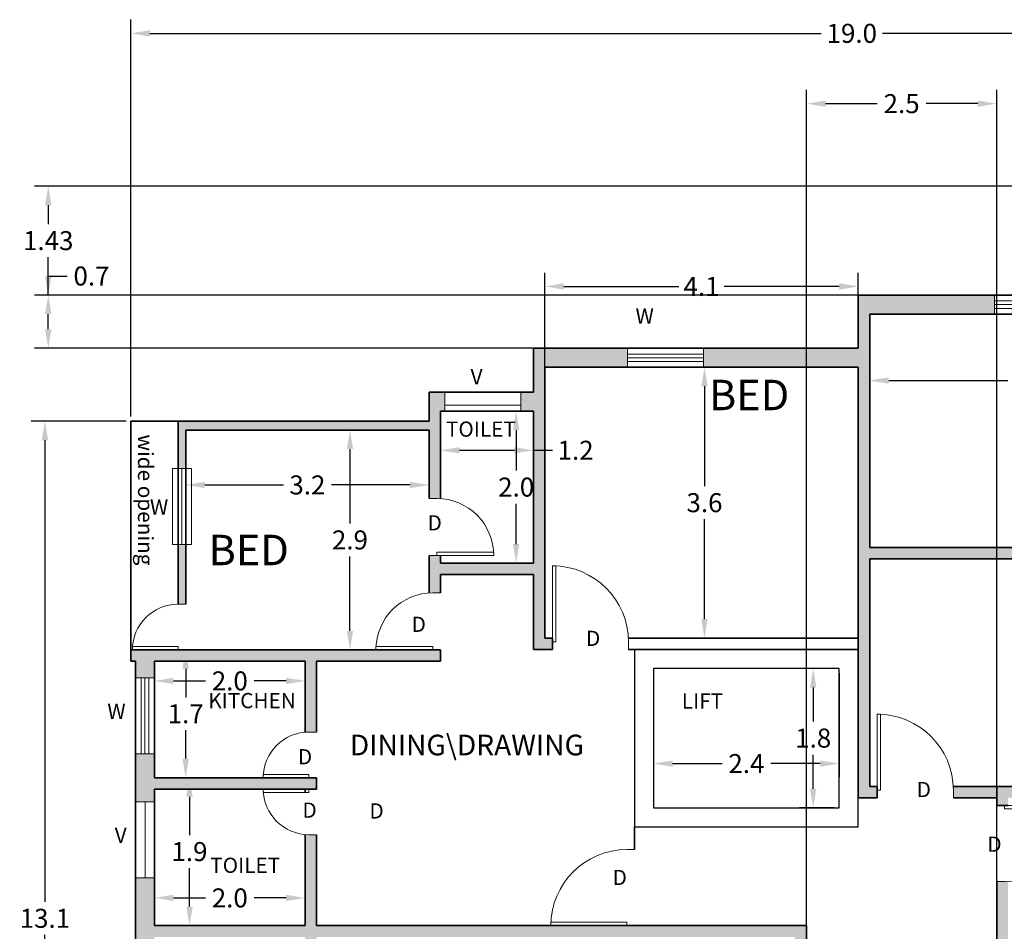
# Model space of a CAD drawing. Units: metres. Extents: x 6.2 to 29.4, y -2.1 to 16.8.
# Tile 2 of 3: x 6.2 to 19.2, y 4.8 to 16.8. Entities that reach past the tile are written whole.
import ezdxf

# ---------------------------------------------------------------- set-up
doc = ezdxf.new("R2010")
doc.units = ezdxf.units.M
doc.header["$MEASUREMENT"] = 0
doc.layers.get('0').update_dxf_attribs({"color": 2})
doc.layers.get('Defpoints').update_dxf_attribs({"color": 3})
for name, color, linetype, lineweight in [('A-ANNO-DIMS', 6, 'Continuous', 13), ('A-ANNO-TEXT', 7, 'Continuous', 18), ('A-AREA-IDEN', 3, 'Continuous', 18), ('A-DOOR', 3, 'Continuous', 18), ('A-EQPM-ELEV', 5, 'Continuous', 25), ('A-GLAZ', 4, 'Continuous', 18), ('A-WALL', 7, 'Continuous', 35), ('A-WALL-PATT', 252, 'Continuous', 13)]:
    doc.layers.add(name, color=color, linetype=linetype, lineweight=lineweight)
doc.styles.get("Standard").update_dxf_attribs({"font": 'arial.ttf'})
doc.dimstyles.get("Standard").update_dxf_attribs({"dimtxt": 0.25, "dimasz": 0.25, "dimexe": 0.18, "dimexo": 0.0625, "dimgap": 0.09, "dimtad": 0, "dimtih": 1, "dimtoh": 1, "dimdec": 1, "dimzin": 0, "dimdsep": 46, "dimtxsty": 'Standard', "dimcen": 0.09, "dimadec": 0, "dimazin": 0, "dimtfac": 1, "dimtdec": 1, "dimtofl": 0, "dimtmove": 0, "dimatfit": 3, "dimfxl": 1, "dimtolj": 1, "dimtzin": 0, "dimarcsym": 0})

# ---------------------------------------------------------------- blocks, each defined once
blk = doc.blocks.new('*U33')
for p, q in [((0, 0), (0, -100)), ((1000, 0), (1000, -100))]:
    blk.add_line(p, q)
blk.add_lwpolyline([(0, 0), (0, 1000), (43.75, 1000), (43.75, 0)], close=True)
blk.add_arc((0, 0), 1000, 0, 90)
blk = doc.blocks.new('*D37')
at = {"layer": 'A-ANNO-DIMS', "color": 0, "lineweight": -2, "transparency": 16777216}
for p, q in [((17.384, 12.84), (17.384, 11.849)), ((21.664, 12.84), (21.664, 11.849)), ((17.634, 12.029), (19.202, 12.029)), ((21.414, 12.029), (19.847, 12.029))]:
    blk.add_line(p, q, dxfattribs=at)
at = {"layer": 'A-ANNO-DIMS', "color": 0, "transparency": 16777216}
for points in [[(17.634, 12.071), (17.634, 11.987), (17.384, 12.029)], [(21.414, 12.071), (21.414, 11.987), (21.664, 12.029)]]:
    blk.add_solid(points, dxfattribs=at)
at = {"layer": 'Defpoints', "color": 0, "transparency": 16777216}
for p in [(17.384, 12.903), (21.664, 12.903), (21.664, 12.029)]:
    blk.add_point(p, dxfattribs=at)
at = {"layer": 'A-ANNO-DIMS', "color": 0, "transparency": 16777216, "insert": (19.524, 12.029), "char_height": 0.25, "attachment_point": 5}
blk.add_mtext('\\A1;4.3', dxfattribs=at)
blk = doc.blocks.new('*D45')
at = {"layer": 'A-ANNO-DIMS', "color": 0, "lineweight": -2, "transparency": 16777216}
for p, q in [((15.237, 12.203), (15.393, 12.203)), ((15.213, 11.953), (15.213, 10.641)), ((15.213, 8.893), (15.213, 10.205)), ((15.237, 8.643), (15.393, 8.643))]:
    blk.add_line(p, q, dxfattribs=at)
at = {"layer": 'A-ANNO-DIMS', "color": 0, "transparency": 16777216}
for points in [[(15.171, 11.953), (15.255, 11.953), (15.213, 12.203)], [(15.171, 8.893), (15.255, 8.893), (15.213, 8.643)]]:
    blk.add_solid(points, dxfattribs=at)
at = {"layer": 'Defpoints', "color": 0, "transparency": 16777216}
for p in [(15.174, 12.203), (15.174, 8.643), (15.213, 8.643)]:
    blk.add_point(p, dxfattribs=at)
at = {"layer": 'A-ANNO-DIMS', "color": 0, "transparency": 16777216, "insert": (15.213, 10.423), "char_height": 0.25, "attachment_point": 5}
blk.add_mtext('\\A1;3.6', dxfattribs=at)
blk = doc.blocks.new('*D46')
at = {"layer": 'A-ANNO-DIMS', "color": 0, "lineweight": -2, "transparency": 16777216}
for p, q in [((13.114, 10.485), (13.114, 13.446)), ((17.234, 12.865), (17.234, 13.446)), ((13.364, 13.266), (14.876, 13.266)), ((16.984, 13.266), (15.473, 13.266))]:
    blk.add_line(p, q, dxfattribs=at)
at = {"layer": 'A-ANNO-DIMS', "color": 0, "transparency": 16777216}
for points in [[(13.364, 13.308), (13.364, 13.224), (13.114, 13.266)], [(16.984, 13.308), (16.984, 13.224), (17.234, 13.266)]]:
    blk.add_solid(points, dxfattribs=at)
at = {"layer": 'Defpoints', "color": 0, "transparency": 16777216}
for p in [(17.234, 13.266), (17.234, 12.803), (13.114, 10.423)]:
    blk.add_point(p, dxfattribs=at)
at = {"layer": 'A-ANNO-DIMS', "color": 0, "transparency": 16777216, "insert": (15.174, 13.266), "char_height": 0.25, "attachment_point": 5}
blk.add_mtext('\\A1;4.1', dxfattribs=at)
blk = doc.blocks.new('*U17')
for p, q in [((-750, 0), (-750, -100)), ((0, 0), (0, -100))]:
    blk.add_line(p, q)
blk.add_lwpolyline([(0, 0), (0, 750), (-43.75, 750), (-43.75, 0)], close=True)
blk.add_arc((0, 0), 750, 90, 180)
blk = doc.blocks.new('*U47')
for p, q in [((-600, 0), (-600, -100)), ((0, 0), (0, -100))]:
    blk.add_line(p, q)
blk.add_lwpolyline([(0, 0), (0, 600), (-43.75, 600), (-43.75, 0)], close=True)
blk.add_arc((0, 0), 600, 90, 180)
blk = doc.blocks.new('*U48')
for p, q in [((0, 0), (0, -100)), ((600, 0), (600, -100))]:
    blk.add_line(p, q)
blk.add_lwpolyline([(0, 0), (0, 600), (43.75, 600), (43.75, 0)], close=True)
blk.add_arc((0, 0), 600, 0, 90)
blk = doc.blocks.new('*D49')
at = {"layer": 'A-ANNO-DIMS', "color": 0, "lineweight": -2, "transparency": 16777216}
for p, q in [((12.712, 11.628), (12.918, 11.628)), ((12.738, 11.378), (12.738, 10.846)), ((12.738, 9.878), (12.738, 10.41)), ((12.712, 9.628), (12.918, 9.628))]:
    blk.add_line(p, q, dxfattribs=at)
at = {"layer": 'A-ANNO-DIMS', "color": 0, "transparency": 16777216}
for points in [[(12.696, 11.378), (12.779, 11.378), (12.738, 11.628)], [(12.696, 9.878), (12.779, 9.878), (12.738, 9.628)]]:
    blk.add_solid(points, dxfattribs=at)
at = {"layer": 'Defpoints', "color": 0, "transparency": 16777216}
for p in [(12.649, 11.628), (12.649, 9.628), (12.738, 9.628)]:
    blk.add_point(p, dxfattribs=at)
at = {"layer": 'A-ANNO-DIMS', "color": 0, "transparency": 16777216, "insert": (12.738, 10.628), "char_height": 0.25, "attachment_point": 5}
blk.add_mtext('\\A1;2.0', dxfattribs=at)
blk = doc.blocks.new('*D50')
at = {"layer": 'A-ANNO-DIMS', "color": 0, "lineweight": -2, "transparency": 16777216}
for p, q in [((11.744, 11.115), (11.744, 11.292)), ((12.964, 11.115), (12.964, 11.292)), ((11.994, 11.112), (12.714, 11.112)), ((12.964, 11.112), (13.214, 11.112))]:
    blk.add_line(p, q, dxfattribs=at)
at = {"layer": 'A-ANNO-DIMS', "color": 0, "transparency": 16777216}
for points in [[(11.994, 11.153), (11.994, 11.07), (11.744, 11.112)], [(12.714, 11.153), (12.714, 11.07), (12.964, 11.112)]]:
    blk.add_solid(points, dxfattribs=at)
at = {"layer": 'Defpoints', "color": 0, "transparency": 16777216}
for p in [(11.744, 11.052), (12.964, 11.112), (12.964, 11.052)]:
    blk.add_point(p, dxfattribs=at)
at = {"layer": 'A-ANNO-DIMS', "color": 0, "transparency": 16777216, "insert": (13.519, 11.112), "char_height": 0.25, "attachment_point": 5}
blk.add_mtext('\\A1;1.2', dxfattribs=at)
blk = doc.blocks.new('*D51')
at = {"layer": 'A-ANNO-DIMS', "color": 0, "lineweight": -2, "transparency": 16777216}
for p, q in [((10.491, 11.378), (10.373, 11.378)), ((10.553, 11.128), (10.553, 10.151)), ((10.553, 8.738), (10.553, 9.715)), ((10.491, 8.488), (10.373, 8.488))]:
    blk.add_line(p, q, dxfattribs=at)
at = {"layer": 'A-ANNO-DIMS', "color": 0, "transparency": 16777216}
for points in [[(10.512, 11.128), (10.595, 11.128), (10.553, 11.378)], [(10.512, 8.738), (10.595, 8.738), (10.553, 8.488)]]:
    blk.add_solid(points, dxfattribs=at)
at = {"layer": 'Defpoints', "color": 0, "transparency": 16777216}
for p in [(10.553, 11.378), (10.553, 8.488), (10.553, 8.488)]:
    blk.add_point(p, dxfattribs=at)
at = {"layer": 'A-ANNO-DIMS', "color": 0, "transparency": 16777216, "insert": (10.553, 9.933), "char_height": 0.25, "attachment_point": 5}
blk.add_mtext('\\A1;2.9', dxfattribs=at)
blk = doc.blocks.new('*D52')
at = {"layer": 'A-ANNO-DIMS', "color": 0, "lineweight": -2, "transparency": 16777216}
for p, q in [((8.394, 10.682), (8.394, 10.476)), ((8.644, 10.656), (9.678, 10.656)), ((11.344, 10.656), (10.31, 10.656)), ((11.594, 10.682), (11.594, 10.476))]:
    blk.add_line(p, q, dxfattribs=at)
at = {"layer": 'A-ANNO-DIMS', "color": 0, "transparency": 16777216}
for points in [[(8.644, 10.697), (8.644, 10.614), (8.394, 10.656)], [(11.344, 10.697), (11.344, 10.614), (11.594, 10.656)]]:
    blk.add_solid(points, dxfattribs=at)
at = {"layer": 'Defpoints', "color": 0, "transparency": 16777216}
for p in [(8.394, 10.744), (11.594, 10.744), (11.594, 10.656)]:
    blk.add_point(p, dxfattribs=at)
at = {"layer": 'A-ANNO-DIMS', "color": 0, "transparency": 16777216, "insert": (9.994, 10.656), "char_height": 0.25, "attachment_point": 5}
blk.add_mtext('\\A1;3.2', dxfattribs=at)
blk = doc.blocks.new('*D53')
at = {"layer": 'A-ANNO-DIMS', "color": 0, "lineweight": -2, "transparency": 16777216}
for p, q in [((8.332, 8.488), (8.214, 8.488)), ((8.394, 8.238), (8.394, 7.863)), ((8.394, 7.058), (8.394, 7.432)), ((8.332, 6.808), (8.214, 6.808))]:
    blk.add_line(p, q, dxfattribs=at)
at = {"layer": 'A-ANNO-DIMS', "color": 0, "transparency": 16777216}
for points in [[(8.352, 8.238), (8.436, 8.238), (8.394, 8.488)], [(8.352, 7.058), (8.436, 7.058), (8.394, 6.808)]]:
    blk.add_solid(points, dxfattribs=at)
at = {"layer": 'Defpoints', "color": 0, "transparency": 16777216}
for p in [(8.394, 8.488), (8.394, 6.808), (8.394, 6.808)]:
    blk.add_point(p, dxfattribs=at)
at = {"layer": 'A-ANNO-DIMS', "color": 0, "transparency": 16777216, "insert": (8.394, 7.648), "char_height": 0.25, "attachment_point": 5}
blk.add_mtext('\\A1;1.7', dxfattribs=at)
blk = doc.blocks.new('*D54')
at = {"layer": 'A-ANNO-DIMS', "color": 0, "lineweight": -2, "transparency": 16777216}
for p, q in [((7.984, 8.142), (7.984, 8.26)), ((9.964, 8.142), (9.964, 8.26)), ((8.234, 8.08), (8.655, 8.08)), ((9.714, 8.08), (9.293, 8.08))]:
    blk.add_line(p, q, dxfattribs=at)
at = {"layer": 'A-ANNO-DIMS', "color": 0, "transparency": 16777216}
for points in [[(8.234, 8.121), (8.234, 8.038), (7.984, 8.08)], [(9.714, 8.121), (9.714, 8.038), (9.964, 8.08)]]:
    blk.add_solid(points, dxfattribs=at)
at = {"layer": 'Defpoints', "color": 0, "transparency": 16777216}
for p in [(7.984, 8.08), (9.964, 8.08), (9.964, 8.08)]:
    blk.add_point(p, dxfattribs=at)
at = {"layer": 'A-ANNO-DIMS', "color": 0, "transparency": 16777216, "insert": (8.974, 8.08), "char_height": 0.25, "attachment_point": 5}
blk.add_mtext('\\A1;2.0', dxfattribs=at)
blk = doc.blocks.new('*D55')
at = {"layer": 'A-ANNO-DIMS', "color": 0, "lineweight": -2, "transparency": 16777216}
for p, q in [((7.984, 5.29), (7.984, 5.407)), ((9.964, 5.29), (9.964, 5.407)), ((8.234, 5.227), (8.655, 5.227)), ((9.714, 5.227), (9.293, 5.227))]:
    blk.add_line(p, q, dxfattribs=at)
at = {"layer": 'A-ANNO-DIMS', "color": 0, "transparency": 16777216}
for points in [[(8.234, 5.269), (8.234, 5.186), (7.984, 5.227)], [(9.714, 5.269), (9.714, 5.186), (9.964, 5.227)]]:
    blk.add_solid(points, dxfattribs=at)
at = {"layer": 'Defpoints', "color": 0, "transparency": 16777216}
for p in [(7.984, 5.227), (9.964, 5.227), (9.964, 5.227)]:
    blk.add_point(p, dxfattribs=at)
at = {"layer": 'A-ANNO-DIMS', "color": 0, "transparency": 16777216, "insert": (8.974, 5.227), "char_height": 0.25, "attachment_point": 5}
blk.add_mtext('\\A1;2.0', dxfattribs=at)
blk = doc.blocks.new('*D56')
at = {"layer": 'A-ANNO-DIMS', "color": 0, "lineweight": -2, "transparency": 16777216}
for p, q in [((8.457, 6.808), (8.624, 6.808)), ((8.444, 6.558), (8.444, 6.053)), ((8.444, 5.113), (8.444, 5.618)), ((8.457, 4.863), (8.624, 4.863))]:
    blk.add_line(p, q, dxfattribs=at)
at = {"layer": 'A-ANNO-DIMS', "color": 0, "transparency": 16777216}
for points in [[(8.403, 6.558), (8.486, 6.558), (8.444, 6.808)], [(8.403, 5.113), (8.486, 5.113), (8.444, 4.863)]]:
    blk.add_solid(points, dxfattribs=at)
at = {"layer": 'Defpoints', "color": 0, "transparency": 16777216}
for p in [(8.394, 6.808), (8.394, 4.863), (8.444, 4.863)]:
    blk.add_point(p, dxfattribs=at)
at = {"layer": 'A-ANNO-DIMS', "color": 0, "transparency": 16777216, "insert": (8.444, 5.836), "char_height": 0.25, "attachment_point": 5}
blk.add_mtext('\\A1;1.9', dxfattribs=at)
blk = doc.blocks.new('*U22')
for p, q in [((0, 0), (0, -100)), ((-1000, 0), (-1000, -100))]:
    blk.add_line(p, q)
blk.add_lwpolyline([(0, 0), (0, 1000), (-43.75, 1000), (-43.75, 0)], close=True)
blk.add_arc((0, 0), 1000, 90, 180)
blk = doc.blocks.new('*D57')
at = {"layer": 'A-ANNO-DIMS', "color": 0, "lineweight": -2, "transparency": 16777216}
for p, q in [((16.922, 8.243), (16.462, 8.243)), ((16.642, 7.993), (16.642, 7.546)), ((16.642, 6.663), (16.642, 7.11)), ((16.922, 6.413), (16.462, 6.413))]:
    blk.add_line(p, q, dxfattribs=at)
at = {"layer": 'A-ANNO-DIMS', "color": 0, "transparency": 16777216}
for points in [[(16.6, 7.993), (16.683, 7.993), (16.642, 8.243)], [(16.6, 6.663), (16.683, 6.663), (16.642, 6.413)]]:
    blk.add_solid(points, dxfattribs=at)
at = {"layer": 'Defpoints', "color": 0, "transparency": 16777216}
for p in [(16.984, 8.243), (16.642, 6.413), (16.984, 6.413)]:
    blk.add_point(p, dxfattribs=at)
at = {"layer": 'A-ANNO-DIMS', "color": 0, "transparency": 16777216, "insert": (16.642, 7.328), "char_height": 0.25, "attachment_point": 5}
blk.add_mtext('\\A1;1.8', dxfattribs=at)
blk = doc.blocks.new('*D58')
at = {"layer": 'A-ANNO-DIMS', "color": 0, "lineweight": -2, "transparency": 16777216}
for p, q in [((14.544, 8.18), (14.544, 6.813)), ((16.984, 8.18), (16.984, 6.813)), ((14.794, 6.993), (15.445, 6.993)), ((16.734, 6.993), (16.083, 6.993))]:
    blk.add_line(p, q, dxfattribs=at)
at = {"layer": 'A-ANNO-DIMS', "color": 0, "transparency": 16777216}
for points in [[(14.794, 7.034), (14.794, 6.951), (14.544, 6.993)], [(16.734, 7.034), (16.734, 6.951), (16.984, 6.993)]]:
    blk.add_solid(points, dxfattribs=at)
at = {"layer": 'Defpoints', "color": 0, "transparency": 16777216}
for p in [(14.544, 8.243), (16.984, 8.243), (16.984, 6.993)]:
    blk.add_point(p, dxfattribs=at)
at = {"layer": 'A-ANNO-DIMS', "color": 0, "transparency": 16777216, "insert": (15.764, 6.993), "char_height": 0.25, "attachment_point": 5}
blk.add_mtext('\\A1;2.4', dxfattribs=at)
blk = doc.blocks.new('*D59')
at = {"layer": 'A-ANNO-DIMS', "color": 0, "lineweight": -2, "transparency": 16777216}
for p, q in [((7.674, 11.556), (7.674, 16.773)), ((26.624, 14.646), (26.624, 16.773)), ((7.924, 16.593), (16.746, 16.593)), ((26.374, 16.593), (17.551, 16.593))]:
    blk.add_line(p, q, dxfattribs=at)
at = {"layer": 'A-ANNO-DIMS', "color": 0, "transparency": 16777216}
for points in [[(7.924, 16.634), (7.924, 16.551), (7.674, 16.593)], [(26.374, 16.634), (26.374, 16.551), (26.624, 16.593)]]:
    blk.add_solid(points, dxfattribs=at)
at = {"layer": 'Defpoints', "color": 0, "transparency": 16777216}
for p in [(7.674, 16.593), (26.624, 14.583), (7.674, 11.494)]:
    blk.add_point(p, dxfattribs=at)
at = {"layer": 'A-ANNO-DIMS', "color": 0, "transparency": 16777216, "insert": (17.149, 16.593), "char_height": 0.25, "attachment_point": 5}
blk.add_mtext('\\A1;19.0', dxfattribs=at)
blk = doc.blocks.new('*D60')
at = {"layer": 'A-ANNO-DIMS', "color": 0, "lineweight": -2, "transparency": 16777216}
for p, q in [((7.611, 11.494), (6.364, 11.494)), ((6.544, 11.244), (6.544, 5.176)), ((6.544, -1.327), (6.544, 4.741)), ((7.611, -1.577), (6.364, -1.577))]:
    blk.add_line(p, q, dxfattribs=at)
at = {"layer": 'A-ANNO-DIMS', "color": 0, "transparency": 16777216}
for points in [[(6.502, 11.244), (6.586, 11.244), (6.544, 11.494)], [(6.502, -1.327), (6.586, -1.327), (6.544, -1.577)]]:
    blk.add_solid(points, dxfattribs=at)
at = {"layer": 'Defpoints', "color": 0, "transparency": 16777216}
for p in [(7.674, 11.494), (6.544, -1.577), (7.674, -1.577)]:
    blk.add_point(p, dxfattribs=at)
at = {"layer": 'A-ANNO-DIMS', "color": 0, "transparency": 16777216, "insert": (6.544, 4.959), "char_height": 0.25, "attachment_point": 5}
blk.add_mtext('\\A1;13.1', dxfattribs=at)
blk = doc.blocks.new('WIN-1000')
for p, q in [((0.075, 1), (0.075, 0)), ((0.125, 1), (0.125, 0)), ((0.175, 1), (0.175, 0))]:
    blk.add_line(p, q)
blk.add_lwpolyline([(0, 1), (0.25, 1), (0.25, 0), (0, 0)], close=True)
blk = doc.blocks.new('VENT-1000')
blk.add_line((0.125, 1), (0.125, 0))
blk.add_lwpolyline([(0, 1), (0.25, 1), (0.25, 0), (0, 0)], close=True)
blk = doc.blocks.new('VENT-1000-OFFSET')
blk.add_line((0, 0.075), (1, 0.075))
blk.add_lwpolyline([(0, 0.25), (1, 0.25), (1, 0), (0, 0)], close=True)
blk = doc.blocks.new('*D71')
at = {"layer": 'A-ANNO-DIMS', "color": 0, "lineweight": -2, "transparency": 16777216}
for p, q in [((16.554, 2.436), (16.554, 15.849)), ((19.054, 2.436), (19.054, 15.849)), ((16.804, 15.669), (17.483, 15.669)), ((18.804, 15.669), (18.125, 15.669))]:
    blk.add_line(p, q, dxfattribs=at)
at = {"layer": 'A-ANNO-DIMS', "color": 0, "transparency": 16777216}
for points in [[(16.804, 15.71), (16.804, 15.627), (16.554, 15.669)], [(18.804, 15.71), (18.804, 15.627), (19.054, 15.669)]]:
    blk.add_solid(points, dxfattribs=at)
at = {"layer": 'Defpoints', "color": 0, "transparency": 16777216}
for p in [(19.054, 15.669), (16.554, 2.373), (19.054, 2.373)]:
    blk.add_point(p, dxfattribs=at)
at = {"layer": 'A-ANNO-DIMS', "color": 0, "transparency": 16777216, "insert": (17.804, 15.669), "char_height": 0.25, "attachment_point": 5}
blk.add_mtext('\\A1;2.5', dxfattribs=at)
blk = doc.blocks.new('*D72')
at = {"layer": 'A-ANNO-DIMS', "color": 0, "lineweight": -2, "transparency": 16777216}
for p, q in [((21.602, 14.583), (6.408, 14.583)), ((6.588, 14.333), (6.588, 14.086)), ((6.588, 13.403), (6.588, 13.65)), ((21.602, 13.153), (6.408, 13.153))]:
    blk.add_line(p, q, dxfattribs=at)
at = {"layer": 'A-ANNO-DIMS', "color": 0, "transparency": 16777216}
for points in [[(6.546, 14.333), (6.63, 14.333), (6.588, 14.583)], [(6.546, 13.403), (6.63, 13.403), (6.588, 13.153)]]:
    blk.add_solid(points, dxfattribs=at)
at = {"layer": 'Defpoints', "color": 0, "transparency": 16777216}
for p in [(6.588, 14.583), (21.664, 14.583), (21.664, 13.153)]:
    blk.add_point(p, dxfattribs=at)
at = {"layer": 'A-ANNO-DIMS', "color": 0, "transparency": 16777216, "insert": (6.588, 13.868), "char_height": 0.25, "attachment_point": 5}
blk.add_mtext('\\A1;1.43', dxfattribs=at)
blk = doc.blocks.new('*D73')
at = {"layer": 'A-ANNO-DIMS', "color": 0, "lineweight": -2, "transparency": 16777216}
for p, q in [((6.588, 13.153), (6.588, 13.403)), ((6.588, 13.403), (6.838, 13.403)), ((17.172, 13.153), (6.408, 13.153)), ((6.588, 12.703), (6.588, 12.903)), ((17.172, 12.453), (6.408, 12.453))]:
    blk.add_line(p, q, dxfattribs=at)
at = {"layer": 'A-ANNO-DIMS', "color": 0, "transparency": 16777216}
for points in [[(6.546, 12.903), (6.63, 12.903), (6.588, 13.153)], [(6.546, 12.703), (6.63, 12.703), (6.588, 12.453)]]:
    blk.add_solid(points, dxfattribs=at)
at = {"layer": 'Defpoints', "color": 0, "transparency": 16777216}
for p in [(6.588, 13.153), (17.234, 13.153), (17.234, 12.453)]:
    blk.add_point(p, dxfattribs=at)
at = {"layer": 'A-ANNO-DIMS', "color": 0, "transparency": 16777216, "insert": (7.156, 13.403), "char_height": 0.25, "attachment_point": 5}
blk.add_mtext('\\A1;0.7', dxfattribs=at)

msp = doc.modelspace()

# ---------------------------------------------------------------- hatches: boundary and pattern name
at = {"layer": 'A-WALL-PATT'}
h = msp.add_hatch(dxfattribs=at)
h.set_pattern_fill('BRICK', color=256, scale=0.3)
h.paths.add_polyline_path([(26.024, -0.354), (25.774, -0.354), (25.774, -1.327), (24.478, -1.327), (24.478, -1.577), (26.024, -1.577)])
h.paths.add_polyline_path([(26.024, 2.199), (25.774, 2.199), (25.774, 2.123), (24.325, 2.123, -0.063254), (24.344, 1.973), (24.344, 1.873), (25.774, 1.873), (25.774, 0.646), (26.024, 0.646)])
h.paths.add_polyline_path([(26.624, 4.802), (26.374, 4.802), (26.374, 3.493), (23.373, 3.493, -0.013897), (23.374, 3.443), (23.374, 3.343), (23.494, 3.343), (23.494, 2.123), (23.344, 2.123), (23.344, 2.023, -0.03766), (23.333, 1.873), (23.744, 1.873), (23.744, 1.973), (23.744, 2.123), (23.644, 2.123), (23.644, 3.343), (25.774, 3.343), (25.774, 3.199), (26.024, 3.199), (26.024, 3.343), (26.624, 3.343)])
h.paths.add_polyline_path([(26.624, 6.775), (26.374, 6.775), (26.374, 6.693), (24.244, 6.693), (24.244, 7.065, -0.016681), (24.194, 7.063), (24.094, 7.063), (24.094, 6.693), (19.054, 6.693), (19.054, 6.443), (19.154, 6.443), (19.204, 6.443), (19.204, 6.543), (22.224, 6.543), (22.224, 3.343), (22.474, 3.343), (22.474, 3.443), (22.474, 3.493), (22.374, 3.493), (22.374, 6.543), (26.374, 6.543), (26.374, 5.802), (26.624, 5.802)])
h.paths.add_polyline_path([(26.624, 8.282), (26.374, 8.282), (26.374, 8.063), (24.244, 8.063), (24.244, 8.163), (24.194, 8.163), (24.094, 8.163), (24.094, 7.813), (24.194, 7.813), (24.244, 7.813), (24.244, 7.913), (26.374, 7.913), (26.374, 7.775), (26.624, 7.775)])
h.paths.add_polyline_path([(26.624, 9.85), (26.374, 9.85), (26.374, 9.733), (24.244, 9.733), (24.244, 10.953), (24.344, 10.953), (24.344, 11.003), (24.344, 11.103), (22.814, 11.103), (22.814, 10.953), (24.094, 10.953), (24.094, 8.913), (24.194, 8.913, -0.016681), (24.244, 8.911), (24.244, 9.583), (26.374, 9.583), (26.374, 9.282), (26.624, 9.282)])
h.paths.add_polyline_path([(26.624, 14.583), (24.36, 14.583), (24.36, 14.333), (25.424, 14.333), (25.424, 11.953), (25.524, 11.953, -0.016681), (25.574, 11.951), (25.574, 14.333), (26.374, 14.333), (26.374, 11.103), (25.574, 11.103), (25.574, 11.203), (25.524, 11.203), (25.424, 11.203), (25.424, 11.103), (25.094, 11.103), (25.094, 11.003, -0.016681), (25.092, 10.953), (26.374, 10.953), (26.374, 10.85), (26.624, 10.85)])
h.paths.add_polyline_path([(23.36, 14.583), (21.664, 14.583), (21.664, 13.153), (20.023, 13.153), (20.023, 12.903), (21.664, 12.903), (21.664, 10.568, -0.050382), (21.814, 10.583), (21.914, 10.583), (21.914, 10.953), (22.014, 10.953), (22.014, 11.053), (22.014, 11.103), (21.914, 11.103), (21.914, 14.333), (23.36, 14.333)])
h.paths.add_polyline_path([(19.023, 13.153), (17.234, 13.153), (17.234, 12.453), (15.201, 12.453), (15.201, 12.203), (17.234, 12.203), (17.234, 8.643), (17.234, 6.543), (17.484, 6.543), (17.484, 6.643), (17.484, 6.693), (17.384, 6.693), (17.384, 9.683), (21.914, 9.683), (21.914, 9.833), (21.814, 9.833), (21.064, 9.833), (17.384, 9.833), (17.384, 12.903), (19.023, 12.903)])
h.paths.add_polyline_path([(14.201, 12.453), (12.964, 12.453), (12.964, 11.878), (12.801, 11.878), (12.801, 11.628), (12.964, 11.628), (12.964, 9.628), (11.744, 9.628), (11.744, 9.728), (11.694, 9.728), (11.594, 9.728), (11.594, 9.236, -0.016681), (11.644, 9.238), (11.744, 9.238), (11.744, 9.478), (12.964, 9.478), (12.964, 8.493), (13.214, 8.493), (13.214, 8.593), (13.214, 8.643), (13.114, 8.643), (13.114, 12.203), (14.201, 12.203)])
h.paths.add_polyline_path([(11.801, 11.878), (11.594, 11.878), (11.594, 11.494), (8.294, 11.494), (8.294, 10.872), (8.394, 10.872), (8.394, 11.378), (11.594, 11.378), (11.594, 10.478), (11.694, 10.478, -0.016681), (11.744, 10.476), (11.744, 11.628), (11.801, 11.628)])
h.paths.add_polyline_path([(8.394, 9.872), (8.294, 9.872), (8.294, 9.088), (8.394, 9.088)])
h.paths.add_polyline_path([(7.984, 7.122), (7.734, 7.122), (7.734, 6.491), (7.984, 6.491), (7.984, 6.658), (9.964, 6.658), (10.014, 6.658), (10.114, 6.658), (10.114, 6.808), (10.014, 6.808), (9.414, 6.808), (7.984, 6.808)])
h.paths.add_polyline_path([(7.984, 5.491), (7.734, 5.491), (7.734, 4.503), (7.984, 4.503), (7.984, 4.713), (9.964, 4.713), (9.964, 4.041, -0.016681), (10.014, 4.043), (10.114, 4.043), (10.114, 4.713), (16.404, 4.713), (16.404, 4.613), (16.454, 4.613), (16.554, 4.613), (16.554, 4.863), (10.114, 4.863), (10.114, 6.058), (10.014, 6.058, -0.020861), (9.964, 6.06), (9.964, 4.863), (7.984, 4.863)])
h.paths.add_polyline_path([(10.114, 3.293), (10.014, 3.293), (9.964, 3.293), (9.964, 3.193), (7.984, 3.193), (7.984, 3.503), (7.734, 3.503), (7.734, 2.884), (7.984, 2.884), (7.984, 3.043), (9.964, 3.043), (9.964, 2.943), (10.014, 2.943), (10.114, 2.943)])
h.paths.add_polyline_path([(7.984, 1.673), (10.216, 1.673, -0.013897), (10.214, 1.723), (10.214, 1.823), (10.114, 1.823), (10.114, 2.193), (10.014, 2.193, -0.016681), (9.964, 2.195), (9.964, 1.823), (7.984, 1.823), (7.984, 1.884), (7.734, 1.884), (7.734, 0.646), (7.984, 0.646)])
h.paths.add_polyline_path([(8.755, -1.327), (7.984, -1.327), (7.984, -0.354), (7.734, -0.354), (7.734, -1.577), (8.755, -1.577)])
h.paths.add_polyline_path([(11.615, -1.327), (11.364, -1.327), (11.364, -0.065, -0.020861), (11.314, -0.067), (11.214, -0.067), (11.214, -1.327), (9.755, -1.327), (9.755, -1.577), (11.615, -1.577)])
h.paths.add_polyline_path([(14.209, -1.327), (12.734, -1.327), (12.734, 0.875, -0.015636), (12.684, 0.873), (12.584, 0.873), (12.584, 0.783), (11.364, 0.783), (11.364, 1.823), (11.114, 1.823), (11.114, 1.723), (11.114, 1.673), (11.214, 1.673), (11.214, 0.533), (11.314, 0.533), (11.364, 0.533), (11.364, 0.633), (12.584, 0.633), (12.584, -1.327), (12.227, -1.327), (12.227, -1.577), (14.209, -1.577)])
h.paths.add_polyline_path([(17.304, -1.327), (16.554, -1.327), (16.554, 3.613), (16.454, 3.613, -0.012506), (16.404, 3.614), (16.404, 1.823), (12.584, 1.823), (12.584, 1.673), (12.684, 1.673), (13.484, 1.673), (16.404, 1.673), (16.404, -1.327), (15.209, -1.327), (15.209, -1.577), (17.304, -1.577)])
h.paths.add_polyline_path([(19.32, -1.327), (19.204, -1.327), (19.204, 1.263), (19.054, 1.263), (19.054, -1.327), (18.304, -1.327), (18.304, -1.577), (19.32, -1.577)])
h.paths.add_polyline_path([(23.478, -1.327), (22.244, -1.327), (22.244, 1.873), (22.344, 1.873), (22.344, 2.023), (22.344, 2.123), (22.094, 2.123), (22.094, 1.263), (21.374, 1.263), (21.374, 1.163, -0.016681), (21.372, 1.113), (22.094, 1.113), (22.094, -1.327), (21.86, -1.327), (21.86, -1.577), (23.478, -1.577)])
h.paths.add_polyline_path([(19.204, 5.444, -0.012506), (19.154, 5.443), (19.054, 5.443), (19.054, 1.263), (19.204, 1.263)])
h.paths.add_polyline_path([(19.054, 6.693), (18.483, 6.693, -0.012506), (18.484, 6.643), (18.484, 6.543), (19.054, 6.543)], flags=17)
h.paths.add_polyline_path([(11.744, 8.488), (7.674, 8.488), (7.674, 8.338), (7.734, 8.338), (7.734, 8.122), (7.984, 8.122), (7.984, 8.338), (9.964, 8.338), (9.964, 7.406, -0.020861), (10.014, 7.408), (10.114, 7.408), (10.114, 8.338), (11.744, 8.338)])
h.paths.add_polyline_path([(15.131, 11.42), (16.48, 11.42), (16.48, 12.245), (15.131, 12.245)], flags=9)
h.paths.add_polyline_path([(8.62, 7.608), (9.947, 7.608), (9.947, 8.021), (8.62, 8.021)], flags=24)

# ---------------------------------------------------------------- linework, layer by layer
at = {"layer": 'A-DOOR'}
for p, q in [((7.694, 8.488), (8.394, 8.488)), ((10.894, 8.488), (11.744, 8.488))]:
    msp.add_line(p, q, dxfattribs=at)
at = {"layer": 'A-EQPM-ELEV'}
for points in [[(17.234, 8.493), (14.294, 8.493), (14.294, 6.163), (17.234, 6.163)], [(16.984, 8.243), (14.544, 8.243), (14.544, 6.413), (16.984, 6.413)]]:
    msp.add_lwpolyline(points, close=True, dxfattribs=at)
at = {"layer": 'A-WALL'}
for p, q in [((17.234, 13.153), (17.234, 12.453)), ((17.234, 13.153), (21.664, 13.153)), ((17.384, 12.903), (17.384, 9.833)), ((17.384, 12.903), (21.664, 12.903)), ((12.964, 12.453), (12.964, 11.878)), ((12.964, 12.453), (17.234, 12.453)), ((13.114, 12.203), (13.114, 8.643)), ((13.114, 12.203), (17.234, 12.203)), ((17.234, 12.203), (17.234, 8.643)), ((11.594, 11.878), (11.594, 11.494)), ((11.594, 11.878), (12.964, 11.878)), ((11.744, 11.628), (11.744, 10.476)), ((11.744, 11.628), (12.964, 11.628)), ((12.964, 11.628), (12.964, 9.628)), ((7.674, 11.494), (8.294, 11.494)), ((7.674, 8.348), (7.674, 11.494)), ((8.294, 11.494), (8.294, 9.088)), ((8.294, 11.494), (11.594, 11.494)), ((8.394, 11.378), (8.394, 9.088)), ((8.394, 11.378), (11.594, 11.378)), ((11.594, 11.378), (11.594, 10.478)), ((12.964, 10.053), (12.964, 9.628)), ((11.594, 9.728), (11.594, 9.236)), ((11.744, 9.728), (11.744, 9.628)), ((17.384, 9.833), (21.914, 9.833)), ((11.744, 9.628), (12.964, 9.628)), ((17.384, 9.683), (17.384, 6.693)), ((17.384, 9.683), (21.914, 9.683)), ((11.744, 9.478), (12.964, 9.478)), ((11.744, 9.478), (11.744, 9.238)), ((12.964, 9.478), (12.964, 8.493)), ((17.234, 9.193), (17.234, 6.543)), ((13.114, 8.643), (13.214, 8.643)), ((13.214, 8.643), (13.214, 8.493)), ((14.213, 8.643), (17.234, 8.643)), ((11.744, 8.488), (7.674, 8.488)), ((11.744, 8.488), (11.744, 8.338)), ((12.964, 8.493), (13.214, 8.493)), ((14.214, 8.493), (17.234, 8.493)), ((7.674, 8.338), (7.674, 8.361)), ((7.734, 8.338), (7.674, 8.338)), ((7.734, -1.577), (7.734, 8.338)), ((7.984, 8.338), (9.964, 8.338)), ((7.984, 6.808), (7.984, 8.338)), ((9.964, 7.406), (9.964, 8.338)), ((10.114, 8.338), (11.744, 8.338)), ((10.114, 7.408), (10.114, 8.338)), ((7.984, 6.808), (9.964, 6.808)), ((9.964, 6.808), (10.114, 6.808)), ((10.114, 6.658), (10.114, 6.808)), ((7.984, 4.863), (7.984, 6.658)), ((7.984, 6.658), (9.964, 6.658)), ((9.964, 6.658), (10.114, 6.658)), ((9.964, 6.614), (9.964, 6.658)), ((17.484, 6.693), (17.384, 6.693)), ((17.484, 6.693), (17.484, 6.543)), ((24.094, 6.693), (18.483, 6.693)), ((19.054, 6.443), (19.054, 6.693)), ((17.484, 6.543), (17.234, 6.543)), ((19.054, 6.543), (18.484, 6.543)), ((19.204, 6.443), (19.054, 6.443)), ((14.294, 6.163), (14.294, 5.863)), ((9.964, 4.863), (9.964, 6.06)), ((10.114, 4.863), (10.114, 6.058)), ((19.054, -1.327), (19.054, 5.443)), ((9.964, 4.863), (7.984, 4.863)), ((16.554, 4.863), (10.114, 4.863)), ((16.554, 4.613), (16.554, 4.863))]:
    msp.add_line(p, q, dxfattribs=at)

# ---------------------------------------------------------------- block references
at = {"layer": 'A-DOOR', "yscale": 0.001, "zscale": 0.001}
for name, p, xscale, rotation in [('*U17', (11.694, 9.728), 0.001, 270), ('*U17', (11.644, 8.488), -0.001, 90), ('*U47', (8.294, 8.488), -0.001, 90), ('*U48', (10.014, 6.808), 0.001, 90), ('*U48', (10.014, 6.658), -0.001, 89.99999999999936), ('*U33', (19.154, 6.443), 0.001, 270), ('*U22', (14.194, 4.863), -0.001, 90)]:
    msp.add_blockref(name, p, dxfattribs=dict(at, xscale=xscale, rotation=rotation))
at = {"layer": 'A-DOOR', "xscale": 0.001, "yscale": 0.001, "zscale": 0.001}
for p in [(13.214, 8.593), (17.484, 6.643)]:
    msp.add_blockref('*U33', p, dxfattribs=at)
at = {"layer": 'A-GLAZ', "extrusion": (0, 0, -1), "zscale": -1}
for p, rotation in [((-20.023, 13.152), 270.0000000000004), ((-15.201, 12.452), 270.0000000000003)]:
    msp.add_blockref('WIN-1000', p, dxfattribs=dict(at, rotation=rotation))
at = {"layer": 'A-GLAZ'}
for name, p in [('VENT-1000-OFFSET', (11.801, 11.629)), ('WIN-1000', (8.219, 9.872)), ('WIN-1000', (7.734, 7.122)), ('VENT-1000', (7.735, 5.491))]:
    msp.add_blockref(name, p, dxfattribs=at)

# ---------------------------------------------------------------- texts
at = {"layer": 'A-ANNO-TEXT', "char_height": 0.2, "attachment_point": 1}
for s, insert in [('W ', (14.307, 12.977)), ('V ', (12.139, 12.179)), ('W ', (7.925, 10.465)), ('D ', (11.574, 10.258)), ('D ', (11.364, 8.924)), ('D ', (13.656, 8.74)), ('W ', (7.365, 7.78)), ('D ', (9.869, 7.183)), ('D ', (18.002, 6.752)), ('D ', (9.929, 6.481)), ('D ', (10.81, 6.471)), ('V ', (7.462, 6.151)), ('D ', (18.931, 6.034)), ('D ', (14.006, 5.596))]:
    msp.add_mtext_dynamic_manual_height_columns(s, width=0.50508, gutter_width=1, heights=[0], dxfattribs=dict(at, insert=insert))
at = {"layer": 'A-ANNO-TEXT', "insert": (7.967, 11.321), "char_height": 0.2, "attachment_point": 1, "rotation": 270}
msp.add_mtext_dynamic_manual_height_columns('wide opening ', width=1.75473, gutter_width=1, heights=[0], dxfattribs=at)
at = {"layer": 'A-AREA-IDEN', "attachment_point": 1}
for s, width, gutter_width, insert, char_height in [('BED', 1.14866, 1, (15.272, 12.039), 0.4), ('TOILET', 1.14866, 1, (11.815, 11.49), 0.2), ('BED', 1.14866, 1, (8.695, 10.001), 0.4), ('KITCHEN', 0.72932, 1, (8.691, 7.921), 0.2), ('LIFT', 1.26548, 1, (14.915, 7.915), 0.2), ('DINING\\\\DRAWING', 2.52682, 1.356, (10.552, 7.373), 0.27123), ('TOILET', 1.14866, 1, (8.717, 5.756), 0.2)]:
    msp.add_mtext_dynamic_manual_height_columns(s, width=width, gutter_width=gutter_width, heights=[0], dxfattribs=dict(at, insert=insert, char_height=char_height))

# ---------------------------------------------------------------- dimensions: what is measured, and where the dimension line sits
at = {"layer": 'A-ANNO-DIMS'}
for base, p1, p2, override, picture, middle in [((7.6735, 16.5927), (26.6241, 14.5831), (7.6735, 11.4939), {"dimclrd": 0, "dimclre": 0, "dimclrt": 0}, '*D59', (17.1488, 16.5927)), ((19.054, 15.669), (16.554, 2.373), (19.054, 2.373), {"dimdec": 1, "dimlfac": 1, "dimrnd": 0, "dimzin": 0, "dimdsep": 46, "dimlunit": 2}, '*D71', (17.804, 15.669)), ((17.234, 13.266), (13.114, 10.423), (17.234, 12.803), {"dimclrd": 0, "dimclre": 0, "dimclrt": 0}, '*D46', (15.174, 13.266)), ((21.664, 12.029), (17.384, 12.903), (21.664, 12.903), {"dimclrd": 0, "dimclre": 0, "dimclrt": 0}, '*D37', (19.524, 12.029)), ((12.964, 11.112), (11.744, 11.052), (12.964, 11.052), {"dimclrd": 0, "dimclre": 0, "dimclrt": 0}, '*D50', (13.519, 11.112)), ((11.594, 10.656), (8.394, 10.744), (11.594, 10.744), {"dimclrd": 0, "dimclre": 0, "dimclrt": 0}, '*D52', (9.994, 10.656)), ((9.964, 8.08), (7.984, 8.08), (9.964, 8.08), {"dimclrd": 0, "dimclre": 0, "dimclrt": 0}, '*D54', (8.974, 8.08)), ((16.984, 6.993), (14.544, 8.243), (16.984, 8.243), {"dimclrd": 0, "dimclre": 0, "dimclrt": 0}, '*D58', (15.764, 6.993)), ((9.964, 5.227), (7.984, 5.227), (9.964, 5.227), {"dimclrd": 0, "dimclre": 0, "dimclrt": 0}, '*D55', (8.974, 5.227))]:
    dim = msp.add_linear_dim(base=base, p1=p1, p2=p2, dimstyle='Standard', override=override, dxfattribs=at)
    dim.commit()
    dim.dimension.update_dxf_attribs({"geometry": picture, "text_midpoint": middle})
for base, p1, p2, override, picture, middle in [((6.588, 14.583), (21.664, 13.153), (21.664, 14.583), {"dimdec": 2, "dimlfac": 1, "dimrnd": 0, "dimzin": 0, "dimdsep": 46, "dimlunit": 2}, '*D72', (6.588, 13.868)), ((6.588, 13.153), (17.234, 12.453), (17.234, 13.153), {"dimdec": 1, "dimlfac": 1, "dimrnd": 0, "dimzin": 0, "dimdsep": 46, "dimlunit": 2}, '*D73', (7.156, 13.403)), ((15.213, 8.643), (15.174, 12.203), (15.174, 8.643), {"dimclrd": 0, "dimclre": 0, "dimclrt": 0}, '*D45', (15.213, 10.423)), ((12.738, 9.628), (12.649, 11.628), (12.649, 9.628), {"dimclrd": 0, "dimclre": 0, "dimclrt": 0}, '*D49', (12.738, 10.628)), ((6.544, -1.577), (7.674, 11.494), (7.674, -1.577), {"dimclrd": 0, "dimclre": 0, "dimclrt": 0}, '*D60', (6.544, 4.959)), ((10.553, 8.488), (10.553, 11.378), (10.553, 8.488), {"dimclrd": 0, "dimclre": 0, "dimclrt": 0}, '*D51', (10.553, 9.933)), ((8.394, 6.808), (8.394, 8.488), (8.394, 6.808), {"dimclrd": 0, "dimclre": 0, "dimclrt": 0}, '*D53', (8.394, 7.648)), ((16.642, 6.413), (16.984, 8.243), (16.984, 6.413), {"dimclrd": 0, "dimclre": 0, "dimclrt": 0}, '*D57', (16.642, 7.328)), ((8.444, 4.863), (8.394, 6.808), (8.394, 4.863), {"dimclrd": 0, "dimclre": 0, "dimclrt": 0}, '*D56', (8.444, 5.836))]:
    dim = msp.add_linear_dim(base=base, p1=p1, p2=p2, angle=90, dimstyle='Standard', override=override, dxfattribs=at)
    dim.commit()
    dim.dimension.update_dxf_attribs({"geometry": picture, "text_midpoint": middle})

doc.saveas('drawing.dxf')
